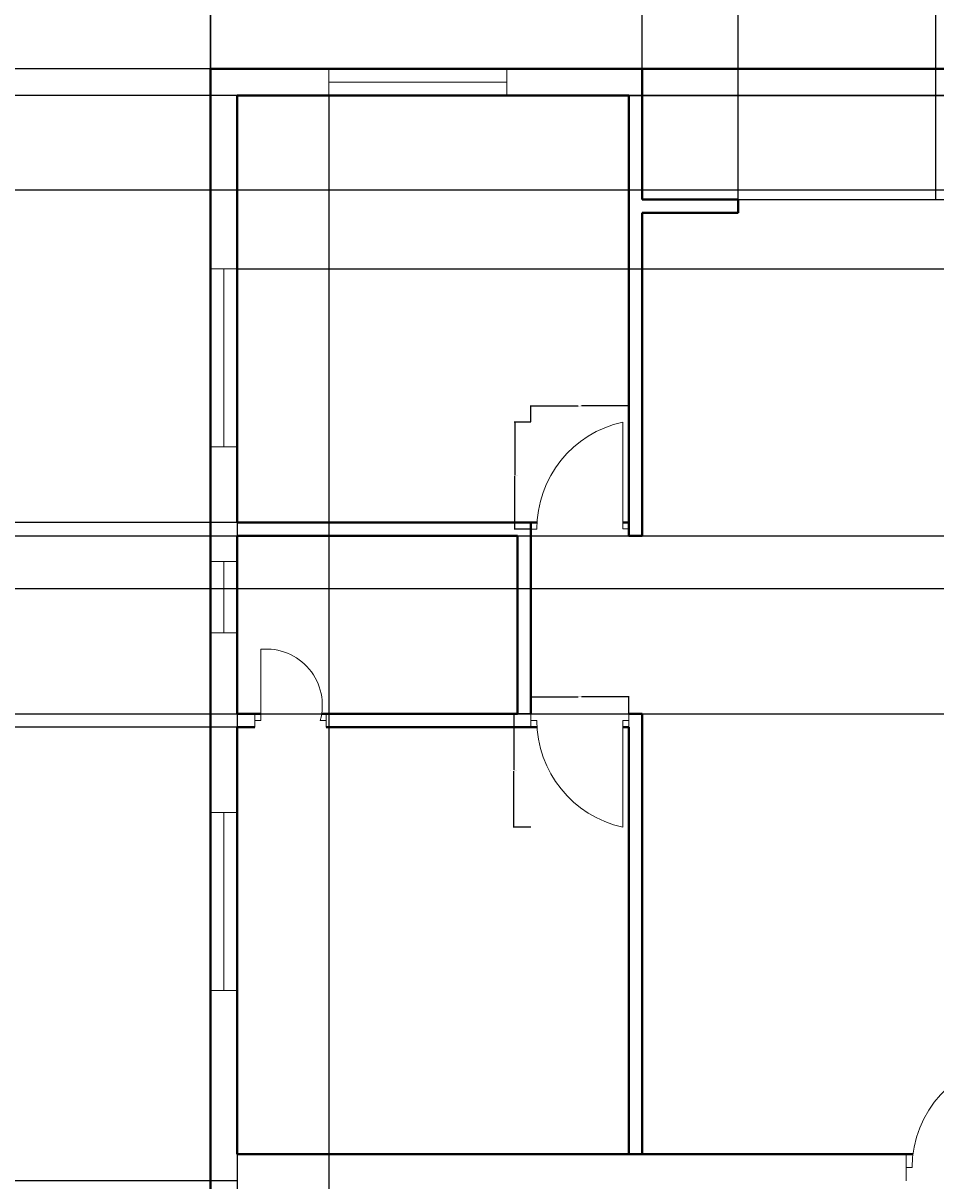
# Model space of a CAD drawing. Units: inches. Extents: x 1355 to 2746, y 1171 to 2751.
# Tile 16 of 24: x 2017 to 2325, y 1764 to 2155. Entities that reach past the tile are written whole.
import ezdxf

# ---------------------------------------------------------------- set-up
doc = ezdxf.new("R2010")
doc.units = ezdxf.units.IN
for name, color, linetype, lineweight in [('A-ANNO-DIMS', 2, 'Continuous', 18), ('A-DOOR', 3, 'Continuous', 20), ('A-GLAZ', 4, 'Continuous', 18), ('A-WALL', 7, 'Continuous', 40)]:
    doc.layers.add(name, color=color, linetype=linetype, lineweight=lineweight)
doc.styles.get("Standard").update_dxf_attribs({"font": 'arial.ttf'})
doc.dimstyles.get("Standard").update_dxf_attribs({"dimtxt": 0.18, "dimasz": 0.18, "dimexe": 0.18, "dimexo": 0.0625, "dimgap": 0.09, "dimtad": 0, "dimtih": 1, "dimtoh": 1, "dimdec": 4, "dimzin": 0, "dimdsep": 46, "dimtxsty": 'Standard', "dimcen": 0.09, "dimadec": 0, "dimazin": 0, "dimtfac": 1, "dimtdec": 4, "dimtofl": 0, "dimtmove": 0, "dimatfit": 3, "dimfxl": 1, "dimtolj": 1, "dimtzin": 0, "dimarcsym": 0})

# ---------------------------------------------------------------- blocks, each defined once
blk = doc.blocks.new('WINDOW-PLAN-24')
for p, q in [((0, 24), (9, 24)), ((9, 24), (4.5, 24)), ((4.5, 24), (4.5, 0)), ((4.5, 0), (0, 0)), ((0, 0), (9, 0))]:
    blk.add_line(p, q)
blk = doc.blocks.new('WINDOW-PLAN-60')
for p, q in [((0, 60), (9, 60)), ((9, 60), (4.5, 60)), ((4.5, 60), (4.5, 0)), ((4.5, 0), (0, 0)), ((0, 0), (9, 0))]:
    blk.add_line(p, q)
blk = doc.blocks.new('WINDOW-PLAN-60-2')
for p, q in [((4.5, 60), (0, 60)), ((0, 60), (9, 60)), ((4.5, 0), (4.5, 60)), ((9, 0), (0, 0)), ((0, 0), (4.5, 0))]:
    blk.add_line(p, q)
blk = doc.blocks.new('DOOR-WC-01')
for p, q in [((2, 2.25), (2, 26.25)), ((0, 4.5), (0, 0)), ((24.04, 4.5), (24.04, 0)), ((0, 0), (0, 2.25)), ((0, 2.25), (2, 2.25)), ((24.04, 2.25), (22.04, 2.25)), ((24.04, 0), (24.04, 2.25))]:
    blk.add_line(p, q)
blk.add_arc((3.76, 7.35), 18.98, 344.4049, 95.3143)
blk = doc.blocks.new('DOOR-ENTRY-N')
for p, q in [((35.29, 4.5), (35.29, 40.5)), ((0, 9), (0, 0)), ((37.29, 9), (37.29, 0)), ((0, 0), (0, 4.5)), ((0, 4.5), (2, 4.5)), ((37.29, 4.5), (35.29, 4.5)), ((37.29, 0), (37.29, 4.5))]:
    blk.add_line(p, q)
blk.add_arc((38.11, 4.5), 36.11, 94.4716, 180)
blk = doc.blocks.new('DOOR-BED-NW')
for p, q in [((31, 0.16), (31, 36.16)), ((33, 0.16), (31, 0.16)), ((0, 0), (2, 0))]:
    blk.add_line(p, q)
blk.add_arc((39.05, 0), 37.05, 102.5441, 180)
blk = doc.blocks.new('DOOR-BEDROOM-NW')
for p, q in [((0, 38.25), (0, 33.75)), ((0, 33.75), (0, 36)), ((0, 36), (2, 36)), ((33, 36), (31, 36)), ((31, 36), (31, 0)), ((33, 33.75), (33, 38.25))]:
    blk.add_line(p, q)
blk.add_arc((38.85, 36), 36.84, 180, 257.7067)
blk = doc.blocks.new('*D75')
at = {"layer": 'A-ANNO-DIMS', "color": 0, "lineweight": -2, "transparency": 16777216}
for p, q in [((2188.33, 2020.17), (2182.79, 2020.17)), ((2182.97, 2019.99), (2182.97, 2002.27)), ((2182.97, 1984.18), (2182.97, 2001.9)), ((2188.33, 1984), (2182.79, 1984))]:
    blk.add_line(p, q, dxfattribs=at)
at = {"layer": 'A-ANNO-DIMS', "color": 0, "transparency": 16777216}
for points in [[(2182.94, 2019.99), (2183, 2019.99), (2182.97, 2020.17)], [(2182.94, 1984.18), (2183, 1984.18), (2182.97, 1984)]]:
    blk.add_solid(points, dxfattribs=at)
at = {"layer": 'Defpoints', "color": 0, "transparency": 16777216}
for p in [(2182.97, 2020.17), (2188.39, 2020.17), (2188.39, 1984)]:
    blk.add_point(p, dxfattribs=at)
at = {"layer": 'A-ANNO-DIMS', "color": 0, "transparency": 16777216, "insert": (2182.97, 2002.08), "char_height": 0.18, "attachment_point": 5}
blk.add_mtext('\\A1;BED DOOR 36 TYP.', dxfattribs=at)
blk = doc.blocks.new('*D76')
at = {"layer": 'A-ANNO-DIMS', "color": 0, "lineweight": -2, "transparency": 16777216}
for p, q in [((2188.39, 2020.23), (2188.39, 2025.77)), ((2188.57, 2025.59), (2204.36, 2025.59)), ((2221.21, 2025.59), (2205.42, 2025.59)), ((2221.39, 2020.23), (2221.39, 2025.77))]:
    blk.add_line(p, q, dxfattribs=at)
at = {"layer": 'A-ANNO-DIMS', "color": 0, "transparency": 16777216}
for points in [[(2188.57, 2025.62), (2188.57, 2025.56), (2188.39, 2025.59)], [(2221.21, 2025.62), (2221.21, 2025.56), (2221.39, 2025.59)]]:
    blk.add_solid(points, dxfattribs=at)
at = {"layer": 'Defpoints', "color": 0, "transparency": 16777216}
for p in [(2221.39, 2025.59), (2188.39, 2020.17), (2221.39, 2020.17)]:
    blk.add_point(p, dxfattribs=at)
at = {"layer": 'A-ANNO-DIMS', "color": 0, "transparency": 16777216, "insert": (2204.89, 2025.59), "char_height": 0.18, "attachment_point": 5}
blk.add_mtext('\\A1;33 TYP.', dxfattribs=at)
blk = doc.blocks.new('*D81')
at = {"layer": 'A-ANNO-DIMS', "color": 0, "lineweight": -2, "transparency": 16777216}
for p, q in [((2188.33, 1921.8), (2182.47, 1921.8)), ((2182.65, 1921.62), (2182.65, 1902.86)), ((2182.65, 1883.73), (2182.65, 1902.49)), ((2188.33, 1883.55), (2182.47, 1883.55))]:
    blk.add_line(p, q, dxfattribs=at)
at = {"layer": 'A-ANNO-DIMS', "color": 0, "transparency": 16777216}
for points in [[(2182.62, 1921.62), (2182.68, 1921.62), (2182.65, 1921.8)], [(2182.62, 1883.73), (2182.68, 1883.73), (2182.65, 1883.55)]]:
    blk.add_solid(points, dxfattribs=at)
at = {"layer": 'Defpoints', "color": 0, "transparency": 16777216}
for p in [(2182.65, 1921.8), (2188.39, 1921.8), (2188.39, 1883.55)]:
    blk.add_point(p, dxfattribs=at)
at = {"layer": 'A-ANNO-DIMS', "color": 0, "transparency": 16777216, "insert": (2182.65, 1902.68), "char_height": 0.18, "attachment_point": 5}
blk.add_mtext('\\A1;BED DOOR 38 TYP.', dxfattribs=at)
blk = doc.blocks.new('*D82')
at = {"layer": 'A-ANNO-DIMS', "color": 0, "lineweight": -2, "transparency": 16777216}
for p, q in [((2188.39, 1921.86), (2188.39, 1927.72)), ((2188.57, 1927.54), (2204.36, 1927.54)), ((2221.21, 1927.54), (2205.42, 1927.54)), ((2221.39, 1921.86), (2221.39, 1927.72))]:
    blk.add_line(p, q, dxfattribs=at)
at = {"layer": 'A-ANNO-DIMS', "color": 0, "transparency": 16777216}
for points in [[(2188.57, 1927.57), (2188.57, 1927.51), (2188.39, 1927.54)], [(2221.21, 1927.57), (2221.21, 1927.51), (2221.39, 1927.54)]]:
    blk.add_solid(points, dxfattribs=at)
at = {"layer": 'Defpoints', "color": 0, "transparency": 16777216}
for p in [(2221.39, 1927.54), (2188.39, 1921.8), (2221.39, 1921.8)]:
    blk.add_point(p, dxfattribs=at)
at = {"layer": 'A-ANNO-DIMS', "color": 0, "transparency": 16777216, "insert": (2204.89, 1927.54), "char_height": 0.18, "attachment_point": 5}
blk.add_mtext('\\A1;33 TYP.', dxfattribs=at)
blk = doc.blocks.new('*D99')
at = {"layer": 'A-ANNO-DIMS', "color": 0, "lineweight": -2, "transparency": 16777216}
for p, q in [((2080.39, 2139.36), (2080.39, 2716.58)), ((2080.57, 2716.4), (2152.75, 2716.4)), ((2225.71, 2716.4), (2153.53, 2716.4)), ((2225.89, 2139.36), (2225.89, 2716.58))]:
    blk.add_line(p, q, dxfattribs=at)
at = {"layer": 'A-ANNO-DIMS', "color": 0, "transparency": 16777216}
for points in [[(2080.57, 2716.43), (2080.57, 2716.37), (2080.39, 2716.4)], [(2225.71, 2716.43), (2225.71, 2716.37), (2225.89, 2716.4)]]:
    blk.add_solid(points, dxfattribs=at)
at = {"layer": 'Defpoints', "color": 0, "transparency": 16777216}
for p in [(2225.89, 2716.4), (2080.39, 2139.3), (2225.89, 2139.3)]:
    blk.add_point(p, dxfattribs=at)
at = {"layer": 'A-ANNO-DIMS', "color": 0, "transparency": 16777216, "insert": (2153.14, 2716.4), "char_height": 0.18, "attachment_point": 5}
blk.add_mtext('\\A1;145.5', dxfattribs=at)
blk = doc.blocks.new('*D100')
at = {"layer": 'A-ANNO-DIMS', "color": 0, "lineweight": -2, "transparency": 16777216}
for p, q in [((2225.89, 2139.36), (2225.89, 2716.58)), ((2226.07, 2716.4), (2293.11, 2716.4)), ((2360.71, 2716.4), (2293.67, 2716.4)), ((2360.89, 2139.36), (2360.89, 2716.58))]:
    blk.add_line(p, q, dxfattribs=at)
at = {"layer": 'A-ANNO-DIMS', "color": 0, "transparency": 16777216}
for points in [[(2226.07, 2716.43), (2226.07, 2716.37), (2225.89, 2716.4)], [(2360.71, 2716.43), (2360.71, 2716.37), (2360.89, 2716.4)]]:
    blk.add_solid(points, dxfattribs=at)
at = {"layer": 'Defpoints', "color": 0, "transparency": 16777216}
for p in [(2360.89, 2716.4), (2225.89, 2139.3), (2360.89, 2139.3)]:
    blk.add_point(p, dxfattribs=at)
at = {"layer": 'A-ANNO-DIMS', "color": 0, "transparency": 16777216, "insert": (2293.39, 2716.4), "char_height": 0.18, "attachment_point": 5}
blk.add_mtext('\\A1;135', dxfattribs=at)
blk = doc.blocks.new('*D102')
at = {"layer": 'A-ANNO-DIMS', "color": 0, "lineweight": -2, "transparency": 16777216}
for p, q in [((2089.33, 1764.3), (1407.53, 1764.3)), ((1407.71, 1764.12), (1407.71, 1725.48)), ((1407.71, 1686.48), (1407.71, 1725.12)), ((2089.33, 1686.3), (1407.53, 1686.3))]:
    blk.add_line(p, q, dxfattribs=at)
at = {"layer": 'A-ANNO-DIMS', "color": 0, "transparency": 16777216}
for points in [[(1407.68, 1764.12), (1407.74, 1764.12), (1407.71, 1764.3)], [(1407.68, 1686.48), (1407.74, 1686.48), (1407.71, 1686.3)]]:
    blk.add_solid(points, dxfattribs=at)
at = {"layer": 'Defpoints', "color": 0, "transparency": 16777216}
for p in [(1407.71, 1764.3), (2089.39, 1764.3), (2089.39, 1686.3)]:
    blk.add_point(p, dxfattribs=at)
at = {"layer": 'A-ANNO-DIMS', "color": 0, "transparency": 16777216, "insert": (1407.71, 1725.3), "char_height": 0.18, "attachment_point": 5}
blk.add_mtext('\\A1;78', dxfattribs=at)
blk = doc.blocks.new('*D103')
at = {"layer": 'A-ANNO-DIMS', "color": 0, "lineweight": -2, "transparency": 16777216}
for p, q in [((2089.33, 1917.3), (1407.53, 1917.3)), ((1407.71, 1917.12), (1407.71, 1840.98)), ((1407.71, 1764.48), (1407.71, 1840.62)), ((2089.33, 1764.3), (1407.53, 1764.3))]:
    blk.add_line(p, q, dxfattribs=at)
at = {"layer": 'A-ANNO-DIMS', "color": 0, "transparency": 16777216}
for points in [[(1407.68, 1917.12), (1407.74, 1917.12), (1407.71, 1917.3)], [(1407.68, 1764.48), (1407.74, 1764.48), (1407.71, 1764.3)]]:
    blk.add_solid(points, dxfattribs=at)
at = {"layer": 'Defpoints', "color": 0, "transparency": 16777216}
for p in [(1407.71, 1917.3), (2089.39, 1917.3), (2089.39, 1764.3)]:
    blk.add_point(p, dxfattribs=at)
at = {"layer": 'A-ANNO-DIMS', "color": 0, "transparency": 16777216, "insert": (1407.71, 1840.8), "char_height": 0.18, "attachment_point": 5}
blk.add_mtext('\\A1;153', dxfattribs=at)
blk = doc.blocks.new('*D104')
at = {"layer": 'A-ANNO-DIMS', "color": 0, "lineweight": -2, "transparency": 16777216}
for p, q in [((2089.33, 1986.3), (1407.53, 1986.3)), ((1407.71, 1986.12), (1407.71, 1951.98)), ((1407.71, 1917.48), (1407.71, 1951.62)), ((2089.33, 1917.3), (1407.53, 1917.3))]:
    blk.add_line(p, q, dxfattribs=at)
at = {"layer": 'A-ANNO-DIMS', "color": 0, "transparency": 16777216}
for points in [[(1407.68, 1986.12), (1407.74, 1986.12), (1407.71, 1986.3)], [(1407.68, 1917.48), (1407.74, 1917.48), (1407.71, 1917.3)]]:
    blk.add_solid(points, dxfattribs=at)
at = {"layer": 'Defpoints', "color": 0, "transparency": 16777216}
for p in [(1407.71, 1986.3), (2089.39, 1986.3), (2089.39, 1917.3)]:
    blk.add_point(p, dxfattribs=at)
at = {"layer": 'A-ANNO-DIMS', "color": 0, "transparency": 16777216, "insert": (1407.71, 1951.8), "char_height": 0.18, "attachment_point": 5}
blk.add_mtext('\\A1;69', dxfattribs=at)
blk = doc.blocks.new('*D105')
at = {"layer": 'A-ANNO-DIMS', "color": 0, "lineweight": -2, "transparency": 16777216}
for p, q in [((2080.33, 2139.3), (1407.53, 2139.3)), ((1407.71, 2139.12), (1407.71, 2062.98)), ((1407.71, 1986.48), (1407.71, 2062.62)), ((2089.33, 1986.3), (1407.53, 1986.3))]:
    blk.add_line(p, q, dxfattribs=at)
at = {"layer": 'A-ANNO-DIMS', "color": 0, "transparency": 16777216}
for points in [[(1407.68, 2139.12), (1407.74, 2139.12), (1407.71, 2139.3)], [(1407.68, 1986.48), (1407.74, 1986.48), (1407.71, 1986.3)]]:
    blk.add_solid(points, dxfattribs=at)
at = {"layer": 'Defpoints', "color": 0, "transparency": 16777216}
for p in [(1407.71, 2139.3), (2080.39, 2139.3), (2089.39, 1986.3)]:
    blk.add_point(p, dxfattribs=at)
at = {"layer": 'A-ANNO-DIMS', "color": 0, "transparency": 16777216, "insert": (1407.71, 2062.8), "char_height": 0.18, "attachment_point": 5}
blk.add_mtext('\\A1;153', dxfattribs=at)
blk = doc.blocks.new('*D108')
at = {"layer": 'A-ANNO-DIMS', "color": 0, "lineweight": -2, "transparency": 16777216}
for p, q in [((2089.39, 2130.24), (2089.39, 1171.06)), ((2120.28, 2130.24), (2120.28, 1171.06)), ((2089.57, 1171.24), (2104.44, 1171.24)), ((2120.1, 1171.24), (2105.23, 1171.24))]:
    blk.add_line(p, q, dxfattribs=at)
at = {"layer": 'A-ANNO-DIMS', "color": 0, "transparency": 16777216}
for points in [[(2089.57, 1171.27), (2089.57, 1171.21), (2089.39, 1171.24)], [(2120.1, 1171.27), (2120.1, 1171.21), (2120.28, 1171.24)]]:
    blk.add_solid(points, dxfattribs=at)
at = {"layer": 'Defpoints', "color": 0, "transparency": 16777216}
for p in [(2089.39, 2130.3), (2120.28, 2130.3), (2120.28, 1171.24)]:
    blk.add_point(p, dxfattribs=at)
at = {"layer": 'A-ANNO-DIMS', "color": 0, "transparency": 16777216, "insert": (2104.84, 1171.24), "char_height": 0.18, "attachment_point": 5}
blk.add_mtext('\\A1;30.89', dxfattribs=at)
blk = doc.blocks.new('*D110')
at = {"layer": 'A-ANNO-DIMS', "color": 0, "lineweight": -2, "transparency": 16777216}
for p, q in [((2089.45, 2130.3), (2648.07, 2130.3)), ((2647.89, 2130.12), (2647.89, 2101.25)), ((2647.89, 2072.02), (2647.89, 2100.89)), ((2089.45, 2071.84), (2648.07, 2071.84))]:
    blk.add_line(p, q, dxfattribs=at)
at = {"layer": 'A-ANNO-DIMS', "color": 0, "transparency": 16777216}
for points in [[(2647.86, 2130.12), (2647.92, 2130.12), (2647.89, 2130.3)], [(2647.86, 2072.02), (2647.92, 2072.02), (2647.89, 2071.84)]]:
    blk.add_solid(points, dxfattribs=at)
at = {"layer": 'Defpoints', "color": 0, "transparency": 16777216}
for p in [(2089.39, 2130.3), (2647.89, 2130.3), (2089.39, 2071.84)]:
    blk.add_point(p, dxfattribs=at)
at = {"layer": 'A-ANNO-DIMS', "color": 0, "transparency": 16777216, "insert": (2647.89, 2101.07), "char_height": 0.18, "attachment_point": 5}
blk.add_mtext('\\A1;58.46', dxfattribs=at)
blk = doc.blocks.new('*D111')
at = {"layer": 'A-ANNO-DIMS', "color": 0, "lineweight": -2, "transparency": 16777216}
for p, q in [((2497.33, 2130.3), (1407.53, 2130.3)), ((1407.71, 2130.12), (1407.71, 2114.5)), ((1407.71, 2098.51), (1407.71, 2114.14)), ((2497.33, 2098.33), (1407.53, 2098.33))]:
    blk.add_line(p, q, dxfattribs=at)
at = {"layer": 'A-ANNO-DIMS', "color": 0, "transparency": 16777216}
for points in [[(1407.68, 2130.12), (1407.74, 2130.12), (1407.71, 2130.3)], [(1407.68, 2098.51), (1407.74, 2098.51), (1407.71, 2098.33)]]:
    blk.add_solid(points, dxfattribs=at)
at = {"layer": 'Defpoints', "color": 0, "transparency": 16777216}
for p in [(1407.71, 2130.3), (2497.39, 2130.3), (2497.39, 2098.33)]:
    blk.add_point(p, dxfattribs=at)
at = {"layer": 'A-ANNO-DIMS', "color": 0, "transparency": 16777216, "insert": (1407.71, 2114.32), "char_height": 0.18, "attachment_point": 5}
blk.add_mtext('\\A1;31.97', dxfattribs=at)
blk = doc.blocks.new('*D112')
at = {"layer": 'A-ANNO-DIMS', "color": 0, "lineweight": -2, "transparency": 16777216}
for p, q in [((2258.27, 2095.29), (2258.27, 2716.58)), ((2258.45, 2716.4), (2291.19, 2716.4)), ((2324.72, 2716.4), (2291.98, 2716.4)), ((2324.9, 2095.29), (2324.9, 2716.58))]:
    blk.add_line(p, q, dxfattribs=at)
at = {"layer": 'A-ANNO-DIMS', "color": 0, "transparency": 16777216}
for points in [[(2258.45, 2716.43), (2258.45, 2716.37), (2258.27, 2716.4)], [(2324.72, 2716.43), (2324.72, 2716.37), (2324.9, 2716.4)]]:
    blk.add_solid(points, dxfattribs=at)
at = {"layer": 'Defpoints', "color": 0, "transparency": 16777216}
for p in [(2324.9, 2716.4), (2258.27, 2095.22), (2324.9, 2095.22)]:
    blk.add_point(p, dxfattribs=at)
at = {"layer": 'A-ANNO-DIMS', "color": 0, "transparency": 16777216, "insert": (2291.58, 2716.4), "char_height": 0.18, "attachment_point": 5}
blk.add_mtext('\\A1;66.63', dxfattribs=at)
blk = doc.blocks.new('*D113')
at = {"layer": 'A-ANNO-DIMS', "color": 0, "lineweight": -2, "transparency": 16777216}
for p, q in [((2225.95, 2139.3), (2648.07, 2139.3)), ((2647.89, 2139.12), (2647.89, 2117.44)), ((2647.89, 2095.4), (2647.89, 2117.08)), ((2225.95, 2095.22), (2648.07, 2095.22))]:
    blk.add_line(p, q, dxfattribs=at)
at = {"layer": 'A-ANNO-DIMS', "color": 0, "transparency": 16777216}
for points in [[(2647.86, 2139.12), (2647.92, 2139.12), (2647.89, 2139.3)], [(2647.86, 2095.4), (2647.92, 2095.4), (2647.89, 2095.22)]]:
    blk.add_solid(points, dxfattribs=at)
at = {"layer": 'Defpoints', "color": 0, "transparency": 16777216}
for p in [(2225.89, 2139.3), (2647.89, 2139.3), (2225.89, 2095.22)]:
    blk.add_point(p, dxfattribs=at)
at = {"layer": 'A-ANNO-DIMS', "color": 0, "transparency": 16777216, "insert": (2647.89, 2117.26), "char_height": 0.18, "attachment_point": 5}
blk.add_mtext('\\A1;44.08', dxfattribs=at)
blk = doc.blocks.new('*D126')
at = {"layer": 'A-ANNO-DIMS', "color": 0, "lineweight": -2, "transparency": 16777216}
for p, q in [((2080.39, 2219.34), (2080.39, 1171.06)), ((2506.39, 2219.34), (2506.39, 1171.06)), ((2080.57, 1171.24), (2293.1, 1171.24)), ((2506.21, 1171.24), (2293.68, 1171.24))]:
    blk.add_line(p, q, dxfattribs=at)
at = {"layer": 'A-ANNO-DIMS', "color": 0, "transparency": 16777216}
for points in [[(2080.57, 1171.27), (2080.57, 1171.21), (2080.39, 1171.24)], [(2506.21, 1171.27), (2506.21, 1171.21), (2506.39, 1171.24)]]:
    blk.add_solid(points, dxfattribs=at)
at = {"layer": 'Defpoints', "color": 0, "transparency": 16777216}
for p in [(2080.39, 2219.4), (2506.39, 2219.4), (2506.39, 1171.24)]:
    blk.add_point(p, dxfattribs=at)
at = {"layer": 'A-ANNO-DIMS', "color": 0, "transparency": 16777216, "insert": (2293.39, 1171.24), "char_height": 0.18, "attachment_point": 5}
blk.add_mtext('\\A1;426', dxfattribs=at)
blk = doc.blocks.new('*D136')
at = {"layer": 'A-ANNO-DIMS', "color": 0, "lineweight": -2, "transparency": 16777216}
for p, q in [((1618.27, 1981.8), (2648.07, 1981.8)), ((2647.89, 1981.62), (2647.89, 1951.98)), ((2647.89, 1921.98), (2647.89, 1951.62)), ((1618.27, 1921.8), (2648.07, 1921.8))]:
    blk.add_line(p, q, dxfattribs=at)
at = {"layer": 'A-ANNO-DIMS', "color": 0, "transparency": 16777216}
for points in [[(2647.86, 1981.62), (2647.92, 1981.62), (2647.89, 1981.8)], [(2647.86, 1921.98), (2647.92, 1921.98), (2647.89, 1921.8)]]:
    blk.add_solid(points, dxfattribs=at)
at = {"layer": 'Defpoints', "color": 0, "transparency": 16777216}
for p in [(1618.21, 1981.8), (2647.89, 1981.8), (1618.21, 1921.8)]:
    blk.add_point(p, dxfattribs=at)
at = {"layer": 'A-ANNO-DIMS', "color": 0, "transparency": 16777216, "insert": (2647.89, 1951.8), "char_height": 0.18, "attachment_point": 5}
blk.add_mtext('\\A1;60', dxfattribs=at)
blk = doc.blocks.new('*D139')
at = {"layer": 'A-ANNO-DIMS', "color": 0, "lineweight": -2, "transparency": 16777216}
for p, q in [((1523.77, 1981.8), (2648.07, 1981.8)), ((2647.89, 1981.62), (2647.89, 1973.09)), ((2647.89, 1964.19), (2647.89, 1972.72)), ((1548.66, 1964.01), (2648.07, 1964.01))]:
    blk.add_line(p, q, dxfattribs=at)
at = {"layer": 'A-ANNO-DIMS', "color": 0, "transparency": 16777216}
for points in [[(2647.86, 1981.62), (2647.92, 1981.62), (2647.89, 1981.8)], [(2647.86, 1964.19), (2647.92, 1964.19), (2647.89, 1964.01)]]:
    blk.add_solid(points, dxfattribs=at)
at = {"layer": 'Defpoints', "color": 0, "transparency": 16777216}
for p in [(1523.71, 1981.8), (1548.6, 1964.01), (2647.89, 1964.01)]:
    blk.add_point(p, dxfattribs=at)
at = {"layer": 'A-ANNO-DIMS', "color": 0, "transparency": 16777216, "insert": (2647.89, 1972.9), "char_height": 0.18, "attachment_point": 5}
blk.add_mtext('\\A1;17.795', dxfattribs=at)

msp = doc.modelspace()

# ---------------------------------------------------------------- linework, layer by layer
at = {"layer": 'A-WALL'}
for p, q in [((2080.3909, 2139.3018), (2225.8909, 2139.3018)), ((2080.3909, 2139.3018), (2080.3909, 1311.3018)), ((2225.8909, 2095.2225), (2225.8909, 2139.3018)), ((2225.8909, 2139.3018), (2360.8909, 2139.3018)), ((2089.3909, 2130.3018), (2221.3909, 2130.3018)), ((2089.3909, 2130.3018), (2089.3909, 1986.3018)), ((2221.3909, 2130.3018), (2221.3909, 1981.8018)), ((2225.8909, 2130.3018), (2225.8909, 2095.2225)), ((2225.8909, 2095.2225), (2258.2658, 2095.2225)), ((2258.2658, 2095.2225), (2258.2658, 2090.7225)), ((2225.8909, 2090.7225), (2225.8909, 1981.8018)), ((2258.2658, 2090.7225), (2225.8909, 2090.7225)), ((2089.3909, 1986.3018), (2190.4622, 1986.3018)), ((2188.3909, 1986.3018), (2188.3909, 1921.8018)), ((2219.3909, 1986.3018), (2221.3909, 1986.3018)), ((2089.3909, 1981.8018), (2183.8909, 1981.8018)), ((2089.3909, 1981.8018), (2089.3909, 1921.8018)), ((2183.8909, 1981.8018), (2183.8909, 1921.8018)), ((2221.3909, 1981.8018), (2225.8909, 1981.8018)), ((2089.3909, 1921.8018), (2097.3512, 1921.8018)), ((2117.8728, 1921.8018), (2183.8909, 1921.8018)), ((2221.3909, 1921.8018), (2225.8909, 1921.8018)), ((2225.8909, 1921.8018), (2225.8909, 1773.3018)), ((2089.3909, 1917.3018), (2095.3512, 1917.3018)), ((2089.3909, 1917.3018), (2089.3909, 1773.3018)), ((2119.3896, 1917.3018), (2190.4596, 1917.3018)), ((2219.3909, 1917.3018), (2221.3909, 1917.3018)), ((2221.3909, 1917.3018), (2221.3909, 1773.3018)), ((2089.3909, 1773.3018), (2221.3909, 1773.3018)), ((2221.3909, 1773.3018), (2317.1838, 1773.3018))]:
    msp.add_line(p, q, dxfattribs=at)

# ---------------------------------------------------------------- block references
at = {"layer": 'A-DOOR'}
for name, p in [('DOOR-BED-NW', (2188.3906, 1984.004)), ('DOOR-WC-01', (2095.3516, 1917.302)), ('DOOR-BEDROOM-NW', (2188.3906, 1883.552)), ('DOOR-ENTRY-N', (2314.9026, 1764.302))]:
    msp.add_blockref(name, p, dxfattribs=at)
at = {"layer": 'A-GLAZ', "extrusion": (0, 0, -1), "zscale": -1, "rotation": 270}
msp.add_blockref('WINDOW-PLAN-60', (-2180.28, 2139.302), dxfattribs=at)
at = {"layer": 'A-GLAZ'}
for name, p in [('WINDOW-PLAN-60-2', (2080.3906, 2011.838)), ('WINDOW-PLAN-60', (2080.3906, 1828.496))]:
    msp.add_blockref(name, p, dxfattribs=at)
at = {"layer": 'A-GLAZ', "extrusion": (0, 0, -1), "zscale": -1}
msp.add_blockref('WINDOW-PLAN-24', (-2089.391, 1949.114), dxfattribs=at)

# ---------------------------------------------------------------- dimensions: what is measured, and where the dimension line sits
at = {"layer": 'A-ANNO-DIMS'}
for base, p1, p2, override, picture, middle in [((2225.8909, 2716.3999), (2080.3909, 2139.3018), (2225.8909, 2139.3018), {"dimdec": 1, "dimlfac": 1, "dimrnd": 0, "dimzin": 0, "dimdsep": 46, "dimlunit": 2}, '*D99', (2153.1409, 2716.3999)), ((2360.8909, 2716.3999), (2225.8909, 2139.3018), (2360.8909, 2139.3018), {"dimdec": 0, "dimlfac": 1, "dimrnd": 0, "dimzin": 0, "dimdsep": 46, "dimlunit": 2}, '*D100', (2293.3909, 2716.3999)), ((2324.8959, 2716.3999), (2258.2658, 2095.2225), (2324.8959, 2095.2225), {"dimdec": 2, "dimlfac": 1, "dimrnd": 0, "dimzin": 0, "dimdsep": 46, "dimlunit": 2}, '*D112', (2291.5809, 2716.3999)), ((2506.3909, 1171.2388), (2080.3909, 2219.3999), (2506.3909, 2219.3999), {"dimdec": 0, "dimlfac": 1, "dimrnd": 0, "dimzin": 0, "dimdsep": 46, "dimlunit": 2}, '*D126', (2293.3909, 1171.2388)), ((2120.2797, 1171.2388), (2089.3909, 2130.3018), (2120.2797, 2130.3017), {"dimdec": 2, "dimlfac": 1, "dimrnd": 0, "dimzin": 0, "dimdsep": 46, "dimlunit": 2}, '*D108', (2104.8353, 1171.2388))]:
    dim = msp.add_linear_dim(base=base, p1=p1, p2=p2, dimstyle='Standard', override=override, dxfattribs=at)
    dim.commit()
    dim.dimension.update_dxf_attribs({"geometry": picture, "text_midpoint": middle})
for base, p1, p2, override, picture, middle in [((1407.7083, 2139.3018), (2089.3909, 1986.3018), (2080.3909, 2139.3018), {"dimdec": 0, "dimlfac": 1, "dimrnd": 0, "dimzin": 0, "dimdsep": 46, "dimlunit": 2}, '*D105', (1407.7083, 2062.8018)), ((2647.886, 2139.3018), (2225.8909, 2095.2225), (2225.8909, 2139.3018), {"dimdec": 2, "dimlfac": 1, "dimrnd": 0, "dimzin": 0, "dimdsep": 46, "dimlunit": 2}, '*D113', (2647.886, 2117.2622)), ((1407.7083, 2130.3018), (2497.3909, 2098.3333), (2497.3909, 2130.3018), {"dimdec": 2, "dimlfac": 1, "dimrnd": 0, "dimzin": 0, "dimdsep": 46, "dimlunit": 2}, '*D111', (1407.7083, 2114.3176)), ((2647.886, 2130.3018), (2089.3909, 2071.8385), (2089.3909, 2130.3018), {"dimdec": 2, "dimlfac": 1, "dimrnd": 0, "dimzin": 0, "dimdsep": 46, "dimlunit": 2}, '*D110', (2647.886, 2101.0702)), ((1407.7083, 1986.3018), (2089.3909, 1917.3018), (2089.3909, 1986.3018), {"dimdec": 0, "dimlfac": 1, "dimrnd": 0, "dimzin": 0, "dimdsep": 46, "dimlunit": 2}, '*D104', (1407.7083, 1951.8018)), ((2647.886, 1964.0069), (1523.7083, 1981.8018), (1548.5973, 1964.0069), {"dimdec": 3, "dimlfac": 1, "dimrnd": 0, "dimzin": 0, "dimdsep": 46, "dimlunit": 2}, '*D139', (2647.886, 1972.9044)), ((2647.886, 1981.8018), (1618.2083, 1921.8018), (1618.2083, 1981.8018), {"dimdec": 0, "dimlfac": 1, "dimrnd": 0, "dimzin": 0, "dimdsep": 46, "dimlunit": 2}, '*D136', (2647.886, 1951.8018)), ((1407.7083, 1917.3018), (2089.3909, 1764.3018), (2089.3909, 1917.3018), {"dimdec": 0, "dimlfac": 1, "dimrnd": 0, "dimzin": 0, "dimdsep": 46, "dimlunit": 2}, '*D103', (1407.7083, 1840.8018)), ((1407.7083, 1764.3018), (2089.3909, 1686.3018), (2089.3909, 1764.3018), {"dimdec": 0, "dimlfac": 1, "dimrnd": 0, "dimzin": 0, "dimdsep": 46, "dimlunit": 2}, '*D102', (1407.7083, 1725.3018))]:
    dim = msp.add_linear_dim(base=base, p1=p1, p2=p2, angle=90, dimstyle='Standard', override=override, dxfattribs=at)
    dim.commit()
    dim.dimension.update_dxf_attribs({"geometry": picture, "text_midpoint": middle})
for base, p1, p2, picture, middle in [((2221.3909, 2025.5897), (2188.3909, 2020.1654), (2221.3909, 2020.1654), '*D76', (2204.8909, 2025.5897)), ((2221.3909, 1927.5393), (2188.3909, 1921.8018), (2221.3909, 1921.8018), '*D82', (2204.8909, 1927.5393))]:
    dim = msp.add_linear_dim(base=base, p1=p1, p2=p2, text='<> TYP.', dimstyle='Standard', override={"dimdec": 0, "dimlfac": 1, "dimrnd": 0, "dimzin": 0, "dimdsep": 46, "dimlunit": 2}, dxfattribs=at)
    dim.commit()
    dim.dimension.update_dxf_attribs({"geometry": picture, "text_midpoint": middle})
for base, p1, p2, picture, middle in [((2182.9666, 2020.1654), (2188.3909, 1984.0037), (2188.3909, 2020.1654), '*D75', (2182.9666, 2002.0845)), ((2182.6534, 1921.8018), (2188.3909, 1883.5518), (2188.3909, 1921.8018), '*D81', (2182.6534, 1902.6768))]:
    dim = msp.add_linear_dim(base=base, p1=p1, p2=p2, angle=90, text='BED DOOR <> TYP.', dimstyle='Standard', override={"dimdec": 0, "dimlfac": 1, "dimrnd": 0, "dimzin": 0, "dimdsep": 46, "dimlunit": 2}, dxfattribs=at)
    dim.commit()
    dim.dimension.update_dxf_attribs({"geometry": picture, "text_midpoint": middle})

doc.saveas('drawing.dxf')
